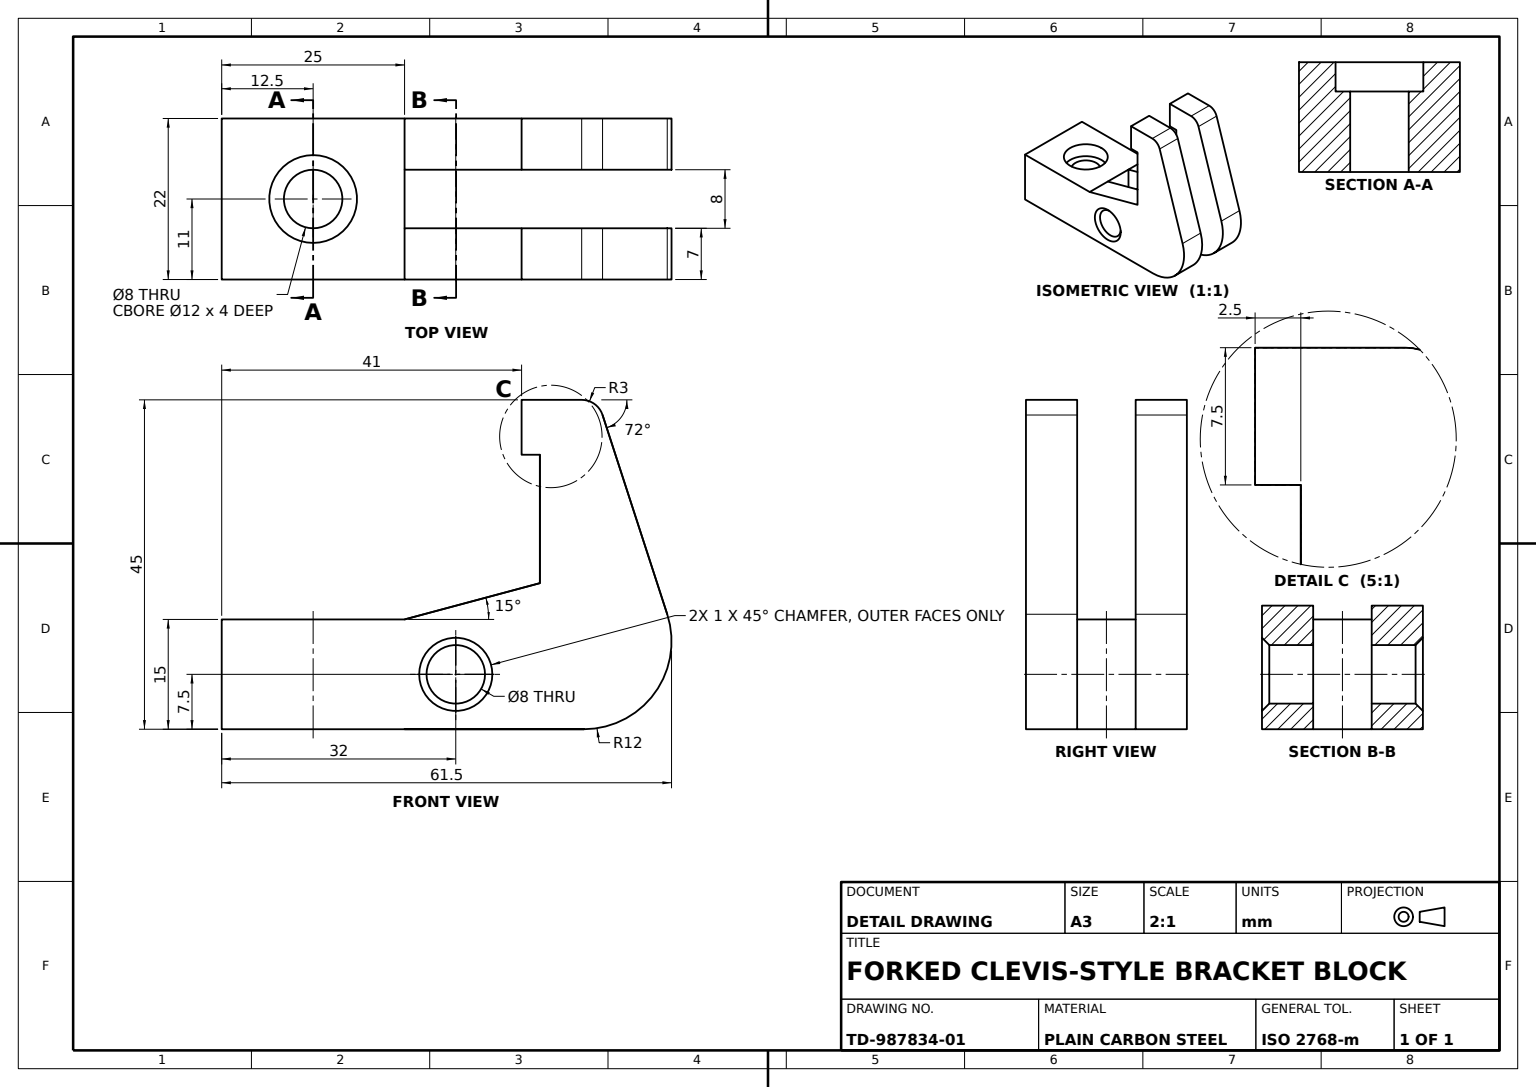
from build123d import *

# Parameters (mm, degrees)
BRACKET_BODY_DEPTH                = 11
FORK_SLOT_SKETCH_W                = 36.5
FORK_SLOT_SKETCH_H                = 8
FORK_SLOT_8MM_DEPTH               = 77.995129716
MOUNTING_HOLE_CBORE_8_D           = 8
MOUNTING_HOLE_CBORE_8_CBORE_D     = 12
MOUNTING_HOLE_CBORE_8_CBORE_DEPTH = 4
CROSS_HOLE_SKETCH_R               = 4
CROSS_HOLE_8_DEPTH                = 80.317400361
CROSS_HOLE_CHAMFER_1MM_SIZE       = 1


with BuildPart() as part:
    # Bracket Profile Sketch → Bracket Body (new, symmetric)
    with BuildSketch(Plane.XY):
        with BuildLine():
            Line((0, 0), (32, 0))
            Line((32, 0), (49.5, 0))
            ThreePointArc((49.5, 0), (59.208203932, 4.946576972), (60.912678196, 15.708203932))
            Line((60.912678196, 15.708203932), (52.06873868, 42.927050983))
            ThreePointArc((52.06873868, 42.927050983), (50.978924888, 44.427050983), (49.215569131, 45))
            Line((49.215569131, 45), (41, 45))
            Line((41, 45), (41, 37.5))
            Line((41, 37.5), (43.5, 37.5))
            Line((43.5, 37.5), (43.5, 19.95706006))
            Line((43.5, 19.95706006), (25, 15))
            Line((25, 15), (0, 15))
            Line((0, 15), (0, 0))
        make_face()
    extrude(amount=BRACKET_BODY_DEPTH, both=True)

    # Fork Slot Sketch → Fork Slot 8mm (cut, through all)
    with BuildSketch(Plane(origin=(0, 0, 0), x_dir=(1, 0, 0), z_dir=(0, 1, 0))):
        with Locations((43.25, 0)):
            Rectangle(FORK_SLOT_SKETCH_W, FORK_SLOT_SKETCH_H)
    extrude(amount=FORK_SLOT_8MM_DEPTH, mode=Mode.SUBTRACT)

    # Mounting Hole CBore Ø8 (through all)
    with Locations(Plane(origin=(12.5, 15, 0), x_dir=(0, 0, 1), z_dir=(0, 1, 0))):
        with Locations((0, 0)):
            CounterBoreHole(MOUNTING_HOLE_CBORE_8_D / 2, MOUNTING_HOLE_CBORE_8_CBORE_D / 2, MOUNTING_HOLE_CBORE_8_CBORE_DEPTH)

    # Cross Hole Sketch → Cross Hole Ø8 (cut, through all)
    with BuildSketch(Plane.XY.offset(11)):
        with Locations((32, 7.5)):
            Circle(CROSS_HOLE_SKETCH_R)
    extrude(amount=-CROSS_HOLE_8_DEPTH, mode=Mode.SUBTRACT)

    # Cross Hole Chamfer 1mm
    cross_hole_chamfer_1mm_edges = [part.edges().sort_by_distance(p)[0] for p in [
        (28, 7.5, -11),
        (28, 7.5, 11),
    ]]
    chamfer(cross_hole_chamfer_1mm_edges, length=CROSS_HOLE_CHAMFER_1MM_SIZE)


solid = part.part
